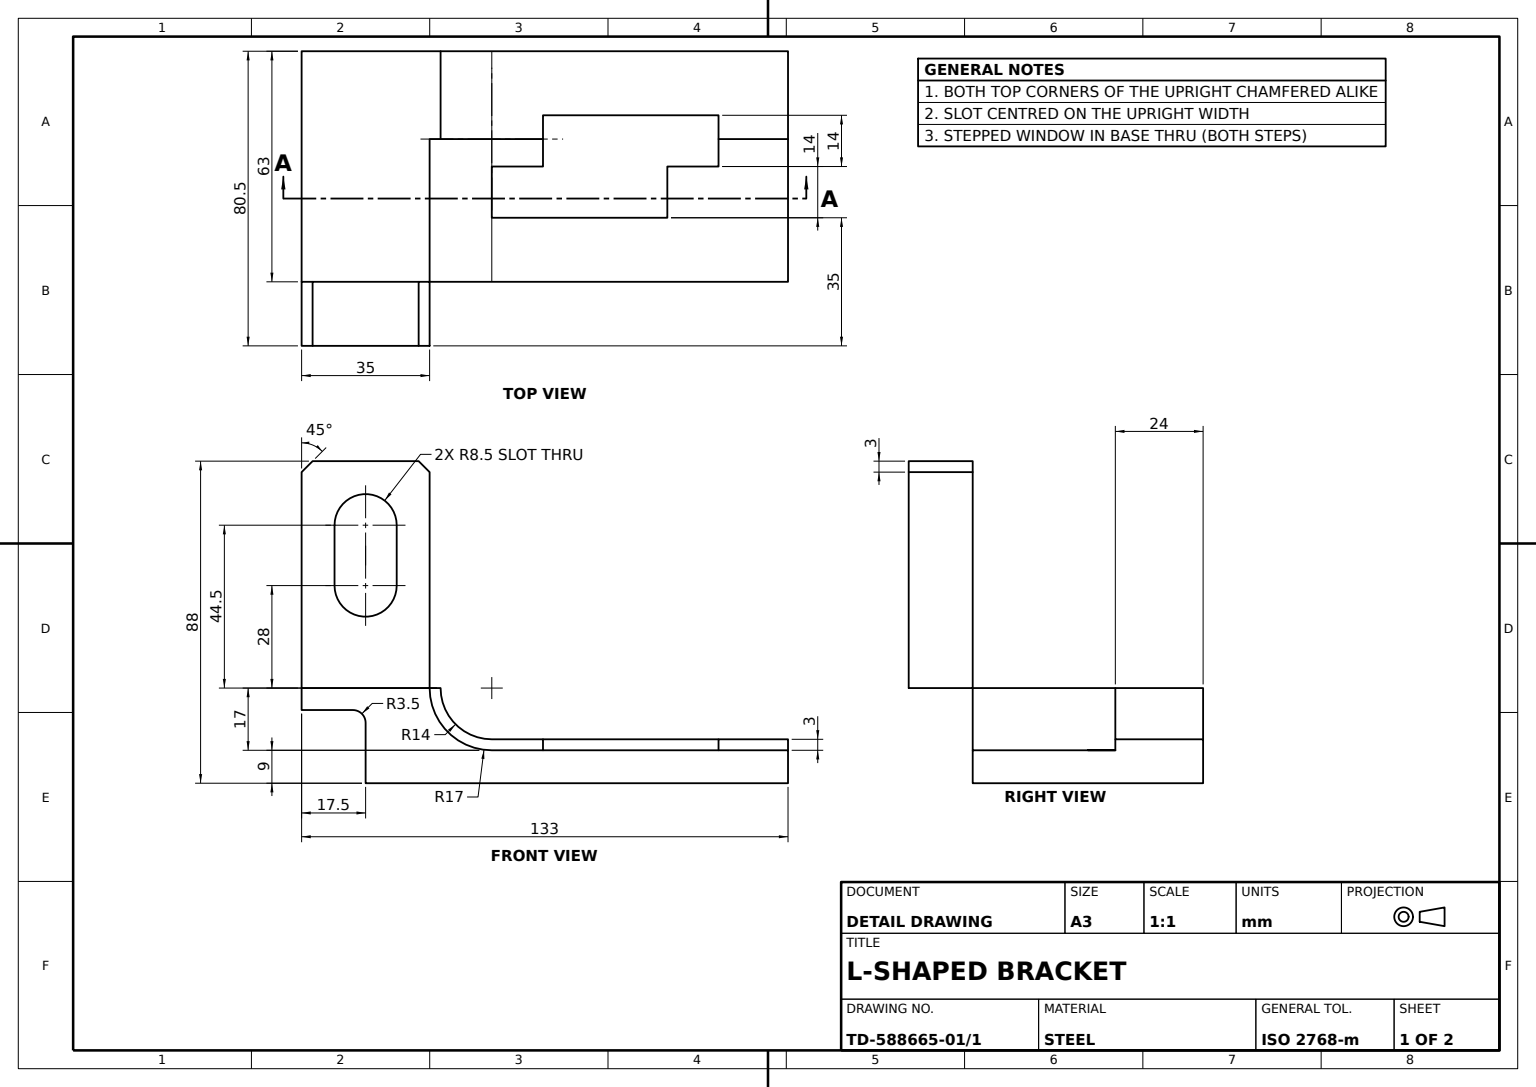
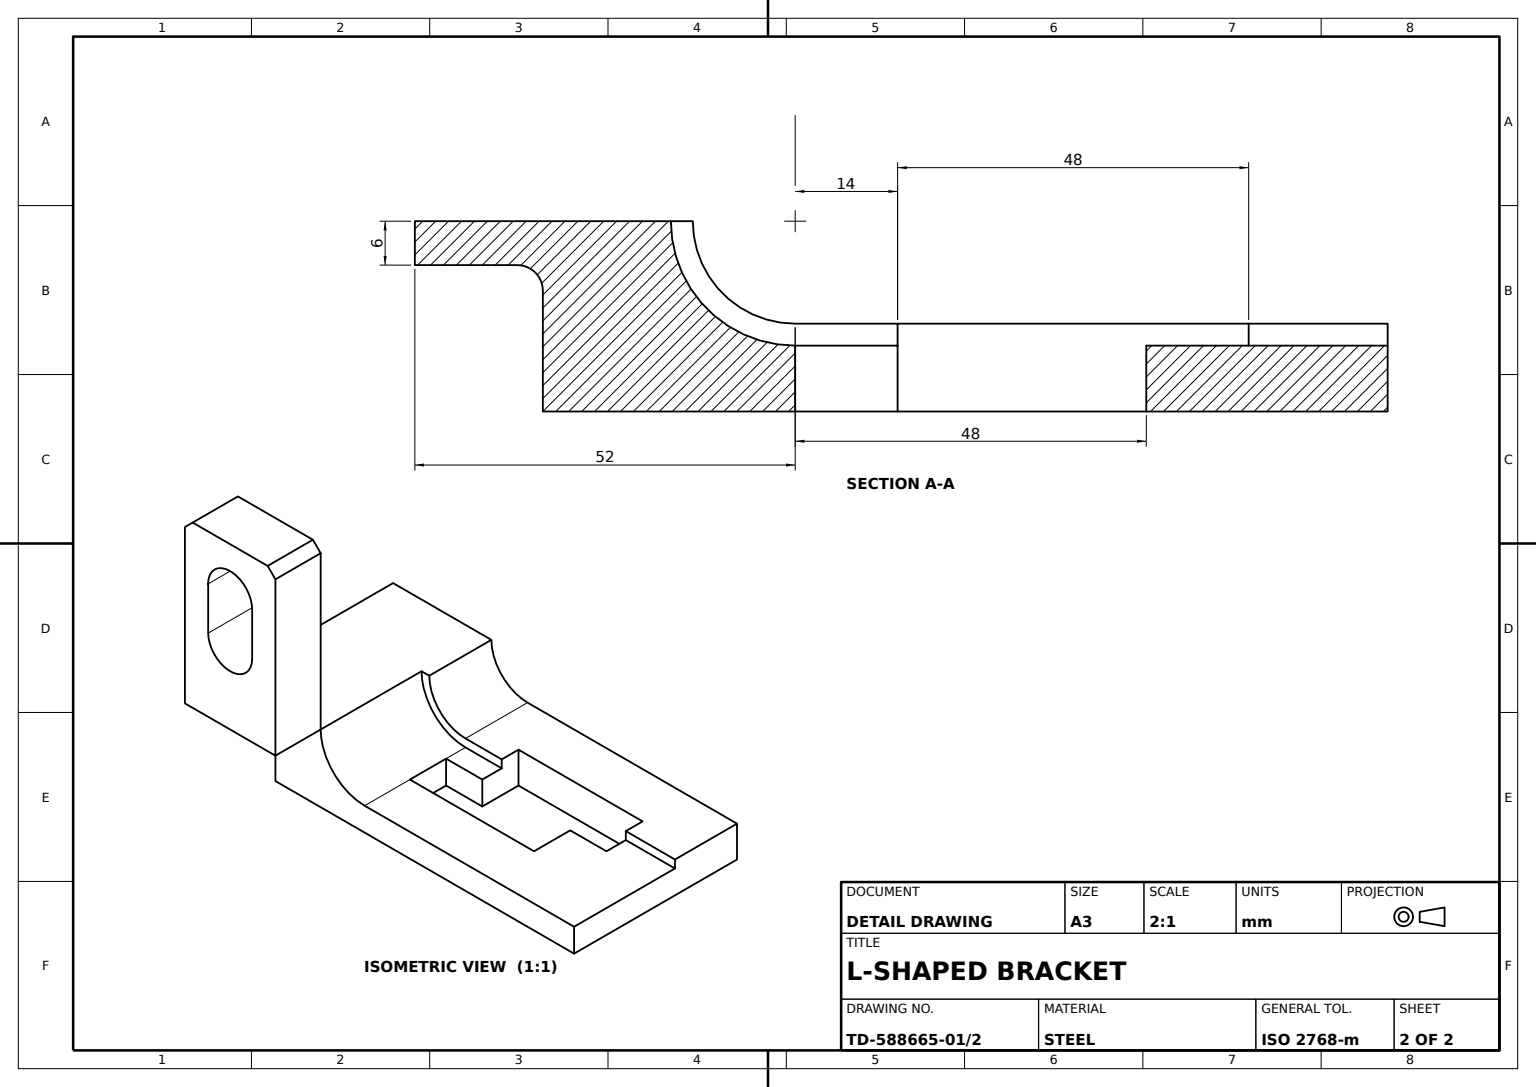
from build123d import *

# Parameters (mm, degrees)
BASE_PLATE_DEPTH           = 63
UPRIGHT_BLOCK_DEPTH        = 17.5
UPRIGHT_OBROUND_SLOT_DEPTH = 17.5
STEPPED_WINDOW_CUT_DEPTH   = 9
RAISED_PAD_DEPTH           = 24
GROOVE_SKETCH_W            = 48
GROOVE_SKETCH_H            = 6.5
GROOVE_CUT_3MM_DEPTH       = 3


with BuildPart() as part:
    # Base Profile Sketch → Base Plate (new body)
    with BuildSketch(Plane.XY):
        with BuildLine():
            Line((0, 0), (115.5, 0))
            Line((115.5, 0), (115.5, 9))
            Line((115.5, 9), (34.5, 9))
            ThreePointArc((34.5, 9), (22.47918472, 13.97918472), (17.5, 26))
            Line((17.5, 26), (-17.5, 26))
            Line((-17.5, 26), (-17.5, 20))
            Line((-17.5, 20), (-3.5, 20))
            ThreePointArc((-3.5, 20), (-1.025126266, 18.974873734), (0, 16.5))
            Line((0, 16.5), (0, 0))
        make_face()
    extrude(amount=BASE_PLATE_DEPTH)

    # Stepped Window Sketch → Stepped Window Cut (cut)
    with BuildSketch(Plane(origin=(0, 9, 0), x_dir=(1, 0, 0), z_dir=(0, 1, 0))):
        Polygon((96.5, -17.5), (48.5, -17.5), (48.5, -31.5), (34.5, -31.5), (34.5, -45.5), (82.5, -45.5), (82.5, -31.5), (96.5, -31.5), align=None)
    extrude(amount=-STEPPED_WINDOW_CUT_DEPTH, mode=Mode.SUBTRACT)

    # Raised Pad Sketch → Raised Pad (add)
    with BuildSketch(Plane(origin=(0, 0, 0), x_dir=(-1, 0, 0), z_dir=(0, 0, -1))):
        with BuildLine():
            Line((-34.5, 12), (-115.5, 12))
            Line((-115.5, 12), (-115.5, 9))
            Line((-115.5, 9), (-34.5, 9))
            ThreePointArc((-34.5, 9), (-22.47918472, 13.97918472), (-17.5, 26))
            Line((-17.5, 26), (-20.5, 26))
            ThreePointArc((-20.5, 26), (-24.600505063, 16.100505063), (-34.5, 12))
        make_face()
    extrude(amount=-RAISED_PAD_DEPTH)

    # Groove Sketch → Groove Cut 3mm (cut)
    with BuildSketch(Plane.XZ.offset(-9)):
        with Locations((72.5, 20.75)):
            Rectangle(GROOVE_SKETCH_W, GROOVE_SKETCH_H)
    extrude(amount=-GROOVE_CUT_3MM_DEPTH, mode=Mode.SUBTRACT)


with BuildPart() as body_2:
    # Upright Block Sketch → Upright Block (new body)
    with BuildSketch(Plane.XY.offset(63)):
        Polygon((0, 26), (17.5, 26), (17.5, 54), (17.5, 70.5), (17.5, 85), (14.5, 88), (0, 88), (-14.5, 88), (-17.5, 85), (-17.5, 26), align=None)
    extrude(amount=UPRIGHT_BLOCK_DEPTH)

    # Upright Slot Sketch → Upright Obround Slot (cut)
    with BuildSketch(Plane.XY.offset(80.5)):
        with BuildLine():
            Line((-8.5, 70.5), (-8.5, 54))
            ThreePointArc((-8.5, 54), (0, 45.5), (8.5, 54))
            Line((8.5, 54), (8.5, 70.5))
            ThreePointArc((8.5, 70.5), (0, 79), (-8.5, 70.5))
        make_face()
    extrude(amount=-UPRIGHT_OBROUND_SLOT_DEPTH, mode=Mode.SUBTRACT)


solid = Compound([part.part, body_2.part])
